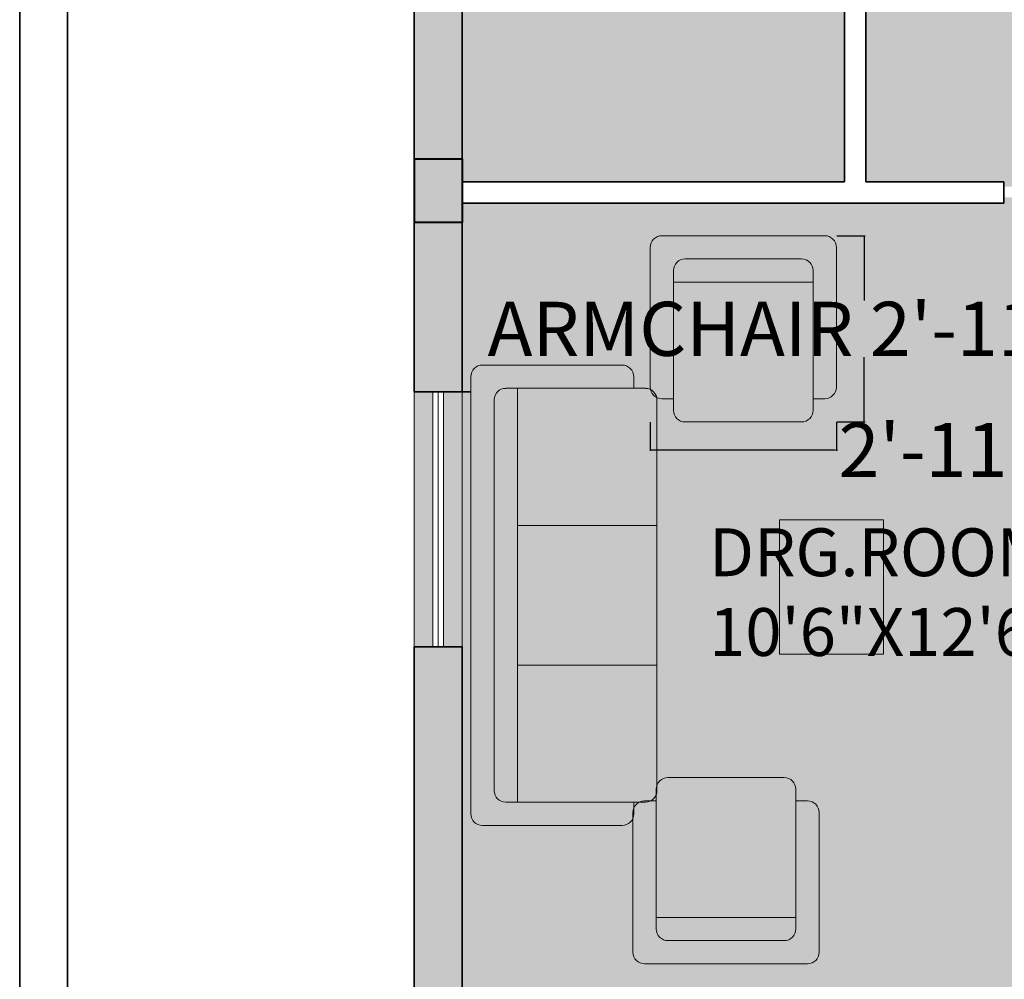
# Model space of a CAD drawing. Units: inches. Extents: x 1077 to 2505, y 1892 to 2728.
# Tile 3 of 26: x 1104 to 1290, y 2157 to 2338. Entities that reach past the tile are written whole.
import ezdxf

# ---------------------------------------------------------------- set-up
doc = ezdxf.new("R2010")
doc.units = ezdxf.units.IN
doc.linetypes.add('ACAD_ISO02W100', pattern=[15, 12, -3])
doc.layers.get('Defpoints').update_dxf_attribs({"color": 220, "linetype": 'ACAD_ISO02W100'})
for name, color, linetype, lineweight in [('00 FURNITURE', 15, 'Continuous', 15), ('A-ANNO-DIMS', 2, 'Continuous', 18), ('A-ANNO-TTLB', 7, 'Continuous', 35), ('A-AREA-IDEN', 7, 'Continuous', 18), ('A-COLS', 7, 'Continuous', 40), ('A-WALL-PATT', 7, 'Continuous', 9), ('WALL', 7, 'Continuous', 35), ('WINDOW', 160, 'Continuous', 13)]:
    doc.layers.add(name, color=color, linetype=linetype, lineweight=lineweight)
doc.layers.add('A-FLOR-PATT', color=254, linetype='Continuous', lineweight=9, true_color=0xd7ebd2)
doc.styles.get("Standard").update_dxf_attribs({"font": 'arial.ttf'})
doc.dimstyles.get("Standard").update_dxf_attribs({"dimtxt": 10.18, "dimasz": 0.18, "dimexe": 0.18, "dimexo": 0.0625, "dimgap": 0.09, "dimtad": 0, "dimtih": 1, "dimtoh": 1, "dimdec": 0, "dimzin": 0, "dimdsep": 46, "dimlunit": 3, "dimtxsty": 'Standard', "dimcen": 0.09, "dimadec": 0, "dimazin": 0, "dimtfac": 1, "dimtdec": 0, "dimtofl": 0, "dimtmove": 0, "dimatfit": 3, "dimfxl": 1, "dimtolj": 1, "dimtzin": 0, "dimarcsym": 0})

# ---------------------------------------------------------------- blocks, each defined once
blk = doc.blocks.new('sofa 6')
for p, q in [((-1044.4, 890), (1044.4, 890)), ((-1100, 166.9), (-1100, 834.3)), ((1100, 834.3), (1100, 166.9)), ((-933.1, 778.7), (933.1, 778.7)), ((-988.8, 55.6), (-988.8, 723.1)), ((988.8, 723.1), (988.8, 55.6)), ((-988.8, 667.5), (988.8, 667.5)), ((-333.8, 667.5), (-333.8, 0)), ((333.7, 667.5), (333.7, 0)), ((-988.8, 111.2), (-1044.4, 111.2)), ((1044.4, 111.2), (988.8, 111.2)), ((933.1, 0), (-933.1, 0))]:
    blk.add_line(p, q)
for centre, start, end in [((-1044.4, 834.3), 90, 180), ((1044.4, 834.3), 0, 90), ((-933.1, 723.1), 90, 180), ((933.1, 723.1), 0, 90), ((-1044.4, 166.9), 180, 270), ((1044.4, 166.9), 270, 0), ((-933.1, 55.6), 180, 270), ((933.1, 55.6), 270, 0)]:
    blk.add_arc(centre, 55.6, start, end)
blk = doc.blocks.new('C1')
h = blk.add_hatch(color=256)
h.dxf.hatch_style = 1
h.paths.add_polyline_path([(1668.56, 2445.41), (1677.56, 2445.41), (1677.56, 2457.41), (1668.56, 2457.41)])
for p, q in [((1668.56, 2457.41), (1677.56, 2457.41)), ((1668.56, 2445.41), (1668.56, 2457.41)), ((1677.56, 2457.41), (1677.56, 2445.41)), ((1677.56, 2445.41), (1668.56, 2445.41))]:
    blk.add_line(p, q)
blk = doc.blocks.new('LOUNGE-ARMCHAIR')
for p, q in [((2.19, 35.04), (32.85, 35.04)), ((0, 6.57), (0, 32.85)), ((35.04, 32.85), (35.04, 6.57)), ((6.57, 30.66), (28.47, 30.66)), ((4.38, 2.19), (4.38, 28.47)), ((30.66, 28.47), (30.66, 2.19)), ((4.38, 26.28), (30.66, 26.28)), ((4.38, 4.38), (2.19, 4.38)), ((32.85, 4.38), (30.66, 4.38)), ((28.47, 0), (6.57, 0))]:
    blk.add_line(p, q)
for centre, start, end in [((2.19, 32.85), 90, 180), ((32.85, 32.85), 0, 90), ((6.57, 28.47), 90, 180), ((28.47, 28.47), 0, 90), ((2.19, 6.57), 180, 270), ((32.85, 6.57), 270, 0), ((6.57, 2.19), 180, 270), ((28.47, 2.19), 270, 0)]:
    blk.add_arc(centre, 2.19, start, end)
blk = doc.blocks.new('WINDOW-48-EXT')
for p, q in [((0, 48), (0, 0)), ((3.5, 48), (3.5, 0)), ((4.5, 48), (4.5, 0)), ((5.5, 48), (5.5, 0)), ((9, 0), (9, 48))]:
    blk.add_line(p, q)
blk = doc.blocks.new('SHEET-FRAME-RESIDENTIAL')
for points in [[(0, 830.04), (543.52, 830.04), (543.52, 0), (0, 0)], [(9, 821.04), (534.52, 821.04), (534.52, 9), (9, 9)]]:
    blk.add_lwpolyline(points, close=True)
blk = doc.blocks.new('*D38')
at = {"layer": 'A-ANNO-DIMS', "color": 0, "lineweight": -2, "transparency": 16777216}
for p, q in [((1258.04, 2297.01), (1263.41, 2297.01)), ((1263.23, 2296.83), (1263.23, 2284.84)), ((1263.23, 2262.15), (1263.23, 2274.13)), ((1258.04, 2261.97), (1263.41, 2261.97))]:
    blk.add_line(p, q, dxfattribs=at)
at = {"layer": 'A-ANNO-DIMS', "color": 0, "transparency": 16777216}
for points in [[(1263.2, 2296.83), (1263.26, 2296.83), (1263.23, 2297.01)], [(1263.2, 2262.15), (1263.26, 2262.15), (1263.23, 2261.97)]]:
    blk.add_solid(points, dxfattribs=at)
at = {"layer": 'Defpoints', "color": 0, "transparency": 16777216}
for p in [(1257.98, 2297.01), (1263.23, 2297.01), (1257.98, 2261.97)]:
    blk.add_point(p, dxfattribs=at)
at = {"layer": 'A-ANNO-DIMS', "color": 0, "transparency": 16777216, "insert": (1263.23, 2279.49), "char_height": 10.18, "attachment_point": 5}
blk.add_mtext('\\A1;ARMCHAIR 2\'-11" TYP.', dxfattribs=at)
blk = doc.blocks.new('*D39')
at = {"layer": 'A-ANNO-DIMS', "color": 0, "lineweight": -2, "transparency": 16777216}
for p, q in [((1222.94, 2261.91), (1222.94, 2256.53)), ((1257.98, 2261.91), (1257.98, 2256.53)), ((1223.12, 2256.71), (1257.8, 2256.71)), ((1257.98, 2256.71), (1258.16, 2256.71))]:
    blk.add_line(p, q, dxfattribs=at)
at = {"layer": 'A-ANNO-DIMS', "color": 0, "transparency": 16777216}
for points in [[(1223.12, 2256.74), (1223.12, 2256.68), (1222.94, 2256.71)], [(1257.8, 2256.74), (1257.8, 2256.68), (1257.98, 2256.71)]]:
    blk.add_solid(points, dxfattribs=at)
at = {"layer": 'Defpoints', "color": 0, "transparency": 16777216}
for p in [(1222.94, 2261.97), (1257.98, 2261.97), (1257.98, 2256.71)]:
    blk.add_point(p, dxfattribs=at)
at = {"layer": 'A-ANNO-DIMS', "color": 0, "transparency": 16777216, "insert": (1293.31, 2256.71), "char_height": 10.18, "attachment_point": 5}
blk.add_mtext('\\A1;2\'-11" TYP.', dxfattribs=at)

msp = doc.modelspace()

# ---------------------------------------------------------------- hatches: boundary and pattern name
at = {"layer": 'A-FLOR-PATT', "transparency": 33554559}
h = msp.add_hatch(color=256, dxfattribs=at)
h.dxf.hatch_style = 1
h.paths.add_polyline_path([(1395.53, 2577.16), (1374.83, 2577.16), (1350.83, 2577.19), (1350.83, 2577.16), (1329.53, 2577.16), (1329.53, 2480.16), (1329.53, 2469.16), (1325.53, 2469.16), (1325.53, 2515.13), (1307.53, 2515.13), (1307.53, 2577.16), (1269.31, 2577.16), (1221.31, 2577.15), (1221.31, 2577.16), (1187.53, 2577.16), (1187.53, 2433.16), (1289.53, 2433.16), (1289.53, 2429.16), (1263.53, 2429.16), (1187.53, 2429.16), (1187.53, 2395.02), (1187.53, 2395.02), (1187.53, 2371.02), (1187.53, 2371.02), (1187.53, 2307.16), (1259.53, 2307.16), (1259.53, 2399.16), (1263.53, 2399.16), (1263.53, 2307.16), (1289.53, 2307.16), (1289.53, 2306.23), (1325.53, 2306.23), (1325.53, 2307.16), (1329.53, 2307.16), (1329.53, 2306.23), (1365.53, 2306.23), (1365.53, 2307.16), (1432.53, 2307.16), (1432.53, 2088.16), (1547.53, 2088.16), (1547.53, 2140.08), (1511.53, 2140.08), (1511.53, 2267.16), (1475.53, 2267.16), (1475.53, 2303.16), (1468.53, 2303.16), (1468.53, 2307.16), (1547.53, 2307.16), (1547.53, 2348.22), (1547.53, 2396.22), (1547.53, 2429.16), (1435.53, 2429.16), (1435.53, 2433.16), (1476.35, 2433.16), (1476.35, 2451.18), (1547.53, 2451.18), (1547.53, 2577.16), (1499.53, 2577.16), (1499.53, 2586.16), (1547.53, 2586.16), (1547.53, 2642.16), (1518.18, 2642.16), (1518.18, 2642.05), (1494.15, 2642.05), (1494.15, 2642.16), (1469.53, 2642.16), (1469.53, 2577.16), (1399.53, 2577.16), (1399.53, 2429.16), (1325.53, 2429.16), (1325.53, 2433.16), (1329.53, 2433.16), (1395.53, 2433.16), (1395.53, 2480.16), (1359.53, 2480.16), (1359.53, 2484.16), (1395.53, 2484.16)])
h.paths.add_polyline_path([(1357.65, 2482.07), (1355.65, 2482.07), (1355.65, 2481.07, 0.414214), (1356.65, 2480.07), (1344.65, 2480.07), (1344.65, 2477.06), (1343.27, 2477.06), (1343.27, 2480.07), (1330.65, 2480.07, -0.414214), (1329.65, 2481.07), (1329.65, 2484.07), (1331.65, 2484.07), (1331.65, 2510.07, -0.446908)], flags=16)
h.paths.add_polyline_path([(1305.09, 2559.18), (1288.89, 2559.18), (1288.89, 2575.38), (1305.09, 2575.38)], flags=16)
h.paths.add_polyline_path([(1304.19, 2560.08), (1289.79, 2560.08), (1289.79, 2574.48), (1304.19, 2574.48)], flags=0)
h.paths.add_polyline_path([(1287.99, 2500.68, -0.414214), (1287.09, 2499.78), (1265.14, 2499.78), (1224.09, 2499.78, -0.414214), (1223.19, 2500.68), (1223.19, 2557.16), (1223.19, 2571.74), (1223.19, 2575.38), (1287.99, 2575.38), (1287.99, 2571.74), (1287.09, 2571.74, -0.414214), (1287.99, 2570.84)], flags=16)
h.paths.add_polyline_path([(1292.98, 2569.05, -1), (1300.92, 2569.05, -1)], flags=0)
h.paths.add_polyline_path([(1293.32, 2569.05, -1), (1300.58, 2569.05, -1)], flags=0)
h.paths.add_polyline_path([(1322.8, 2462.21), (1322.8, 2431.71), (1323.05, 2430.71), (1323.05, 2431.71), (1321.8, 2431.71), (1321.8, 2462.19, 0.404641), (1292.3, 2431.71), (1292.05, 2430.71, -0.414214), (1291.55, 2430.21), (1291.05, 2430.21), (1291.05, 2429.71, -0.414214), (1290.55, 2429.21), (1289.55, 2429.21), (1289.55, 2434.21), (1290.55, 2434.21, -0.414214), (1291.05, 2433.71), (1291.05, 2433.21), (1291.55, 2433.21, -0.414214), (1292.05, 2432.71), (1292.3, 2431.71, -0.414214)], flags=16)
h.paths.add_polyline_path([(1287.82, 2548.28, 0.292232), (1279.17, 2536.8, 0.052719), (1223.93, 2548.28), (1223.28, 2548.28), (1223.28, 2557.16), (1223.93, 2557.16), (1245.42, 2557.16, -0.117785), (1245.77, 2557.93, -0.059418), (1254.87, 2567.02, -0.379859), (1257.28, 2566.88, -0.02509), (1261.41, 2563.32, -0.025935), (1265.65, 2567.02, -0.379859), (1268.06, 2566.88, -0.061767), (1277.52, 2557.43, -0.069393), (1277.82, 2557.16), (1287.82, 2557.16)], flags=0)
h.paths.add_polyline_path([(1263.47, 2548.28), (1260.56, 2548.28, -0.015371), (1258.01, 2546.13, -0.429576), (1255.37, 2546.06, -0.016036), (1252.69, 2548.28), (1223.28, 2548.28), (1223.28, 2554.42), (1246.78, 2554.42, 0.055344), (1255.37, 2546.06, 0.331768), (1257.52, 2545.74, 0.027343), (1262, 2549.64, 0.00919)], flags=0)
h.paths.add_polyline_path([(1295.56, 2568.34), (1296.87, 2569.09), (1296.87, 2570.6, 0.399698), (1295.39, 2569.05, 0.119004)], flags=0)
h.paths.add_polyline_path([(1295.21, 2569.05, -1), (1298.68, 2569.05, -1)], flags=0)
h.paths.add_polyline_path([(1296.95, 2568.96), (1297.03, 2569), (1297.03, 2569.09), (1296.99, 2569.11), (1296.91, 2568.98)], flags=0)
h.paths.add_polyline_path([(1402.28, 2462.19, -0.414214), (1432.78, 2431.69), (1433.03, 2432.69), (1432.78, 2431.69, 0.404641), (1403.28, 2462.17), (1403.28, 2431.69), (1402.03, 2431.69), (1402.03, 2430.69, -0.414214), (1401.53, 2430.19), (1401.03, 2430.19), (1401.03, 2429.69, -0.414214), (1400.53, 2429.19), (1399.53, 2429.19), (1399.53, 2434.19), (1400.53, 2434.19, -0.414214), (1401.03, 2433.69), (1401.03, 2433.19), (1401.53, 2433.19, -0.414214), (1402.03, 2432.69)], flags=16)
h.paths.add_polyline_path([(1470.16, 2535.21, -0.414214), (1471.06, 2536.11), (1527.54, 2536.11), (1542.12, 2536.11), (1545.76, 2536.11), (1545.76, 2471.31), (1542.12, 2471.31), (1542.12, 2472.21, -0.414214), (1541.22, 2471.31), (1471.06, 2471.31, -0.414214), (1470.16, 2472.21), (1470.16, 2494.16)], flags=16)
h.paths.add_polyline_path([(1483.07, 2536.11, 0.253465), (1480.11, 2526.15, 0.2538), (1470.15, 2523.19)], flags=16)
h.paths.add_polyline_path([(1223.19, 2512.69, 0.253465), (1233.14, 2509.74, 0.2538), (1236.1, 2499.77)], flags=16)
h.paths.add_polyline_path([(1469.77, 2578.72), (1469.77, 2581.72), (1471.77, 2581.72), (1471.77, 2607.72, -0.01951), (1473.77, 2607.68), (1473.77, 2579.72), (1473.77, 2578.72, -0.414214), (1472.77, 2577.72), (1470.77, 2577.72, -0.414214)], flags=16)
h.paths.add_polyline_path([(1382.46, 2398.13), (1395.04, 2398.13), (1395.04, 2399.74), (1382.46, 2399.74)], flags=16)
h.paths.add_polyline_path([(1379.94, 2397.18), (1379.94, 2389.82), (1380.5, 2389.82), (1380.5, 2396.05, -0.41429), (1381.06, 2396.61), (1396.47, 2396.61, -0.414213), (1397.03, 2396.05), (1397.03, 2389.82), (1397.59, 2389.82), (1397.59, 2397.18)], flags=16)
h.paths.add_polyline_path([(1263.37, 2428.14), (1263.37, 2426.14, -0.414214), (1262.37, 2425.14), (1261.37, 2425.14), (1233.41, 2425.14, 0.400854), (1259.37, 2401.04), (1259.37, 2401.14), (1261.37, 2401.14, -0.446908), (1233.37, 2427.14), (1259.37, 2427.14), (1259.37, 2429.14), (1262.37, 2429.14, -0.414214)], flags=16)
h.paths.add_polyline_path([(1404.79, 2398.13), (1417.37, 2398.13), (1417.37, 2399.74), (1404.79, 2399.74)], flags=16)
h.paths.add_polyline_path([(1402.27, 2397.18), (1404.79, 2398.13), (1417.37, 2398.13), (1419.92, 2397.18)], flags=16)
h.paths.add_polyline_path([(1432.26, 2383.16), (1432.26, 2370.59), (1433.87, 2370.59), (1433.87, 2383.16)], flags=16)
h.paths.add_polyline_path([(1431.3, 2385.69), (1423.84, 2385.69), (1423.84, 2385.13), (1430.18, 2385.13, -0.41429), (1430.74, 2384.57), (1430.74, 2369.16, -0.414237), (1430.18, 2368.6), (1423.84, 2368.6), (1423.84, 2368.03), (1431.3, 2368.03)], flags=16)
h.paths.add_polyline_path([(1417.37, 2351.16), (1417.37, 2349.54), (1418.9, 2349.54, 0.414236), (1419.92, 2350.56), (1419.92, 2352.11)], flags=16)
h.paths.add_polyline_path([(1395.04, 2351.16), (1395.04, 2349.54), (1396.58, 2349.54, 0.414235), (1397.59, 2350.56), (1397.59, 2352.11)], flags=16)
h.paths.add_polyline_path([(1366.7, 2370.05), (1365.09, 2370.05), (1365.09, 2368.52, 0.414235), (1366.11, 2367.5), (1367.66, 2367.5)], flags=16)
h.paths.add_polyline_path([(1419.36, 2359.47), (1419.36, 2353.24, -0.41419), (1418.8, 2352.68), (1403.39, 2352.68, -0.414137), (1402.83, 2353.24), (1402.83, 2359.47), (1397.03, 2359.47), (1397.03, 2353.24, -0.414189), (1396.47, 2352.68), (1381.06, 2352.68, -0.414137), (1380.5, 2353.24), (1380.5, 2359.47)], flags=16)
h.paths.add_polyline_path([(1222.29, 2559.18), (1206.09, 2559.18), (1206.09, 2575.38), (1222.29, 2575.38)], flags=16)
h.paths.add_polyline_path([(1221.39, 2560.08), (1206.99, 2560.08), (1206.99, 2574.48), (1221.39, 2574.48)], flags=0)
h.paths.add_polyline_path([(1482, 2577.72), (1482, 2580.73), (1483.38, 2580.73), (1483.38, 2577.72), (1484.77, 2577.72), (1484.77, 2574.72), (1483.38, 2574.72), (1483.38, 2577.72)], flags=16)
h.paths.add_polyline_path([(1266.37, 2415.53), (1266.37, 2414.14), (1263.37, 2414.14), (1263.37, 2415.53), (1260.36, 2415.53), (1260.36, 2416.91), (1263.37, 2416.91), (1263.37, 2415.53)], flags=16)
h.paths.add_polyline_path([(1210.26, 2569.05, -1), (1218.19, 2569.05, -1)], flags=0)
h.paths.add_polyline_path([(1210.6, 2569.05, -1), (1217.85, 2569.05, -1)], flags=0)
h.paths.add_polyline_path([(1212.84, 2568.34), (1214.15, 2569.09), (1214.15, 2570.6, 0.399698), (1212.67, 2569.05, 0.119004)], flags=0)
h.paths.add_polyline_path([(1212.49, 2569.05, -1), (1215.96, 2569.05, -1)], flags=0)
h.paths.add_polyline_path([(1214.23, 2568.96), (1214.3, 2568.91), (1214.3, 2569)], flags=0)
h.paths.add_polyline_path([(1507.18, 2480.12, 0.052719), (1518.66, 2535.36), (1518.66, 2536.01), (1527.54, 2536.01), (1527.54, 2535.36), (1527.54, 2513.88, -0.117785), (1528.31, 2513.53, -0.059418), (1537.4, 2504.43, -0.379859), (1537.26, 2502.01, -0.02509), (1533.7, 2497.89, -0.025935), (1537.4, 2493.64, -0.379859), (1537.26, 2491.23, -0.061767), (1527.8, 2481.77, -0.069393), (1527.54, 2481.47), (1527.54, 2471.47), (1518.66, 2471.47, 0.292232)], flags=0)
h.paths.add_polyline_path([(1516.43, 2503.92, -0.016036), (1518.66, 2506.6), (1518.66, 2536.01), (1524.8, 2536.01), (1524.8, 2512.51, 0.055344), (1516.43, 2503.92, 0.331768), (1516.12, 2501.77, 0.027343), (1520.01, 2497.29, 0.00919), (1518.66, 2495.82), (1518.66, 2498.73, -0.015371), (1516.5, 2501.28, -0.429576)], flags=0)
h.paths.add_polyline_path([(1499.63, 2625.5, -0.171636), (1502.82, 2631.01), (1502.82, 2633.37), (1498.68, 2633.37, -0.414214), (1497.7, 2634.36), (1497.7, 2640.66, -0.414214), (1498.68, 2641.64), (1514.82, 2641.64, -0.414214), (1515.81, 2640.66), (1515.81, 2634.36, -0.414214), (1514.82, 2633.37), (1510.69, 2633.37), (1510.69, 2631.01, -0.171636), (1513.88, 2625.5, -0.258205), (1509.31, 2614.47), (1504.19, 2614.47, -0.258205)], flags=16)
h.paths.add_polyline_path([(1501.2, 2625.5, -0.171636), (1504.39, 2631.01), (1509.12, 2631.01, -0.171636), (1512.3, 2625.5, -0.210384), (1509.35, 2616.02), (1504.16, 2616.02, -0.210384)], flags=0)
h.paths.add_polyline_path([(1529.56, 2537.01), (1529.56, 2553.21), (1545.76, 2553.21), (1545.76, 2537.01)], flags=16)
h.paths.add_polyline_path([(1530.46, 2537.91), (1530.46, 2552.31), (1544.86, 2552.31), (1544.86, 2537.91)], flags=0)
h.paths.add_polyline_path([(1535.45, 2545.07, -1), (1543.39, 2545.07, -1)], flags=0)
h.paths.add_polyline_path([(1535.8, 2545.07, -1), (1543.05, 2545.07, -1)], flags=0)
h.paths.add_polyline_path([(1529.56, 2470.41), (1545.76, 2470.41), (1545.76, 2454.21), (1529.56, 2454.21)], flags=16)
h.paths.add_polyline_path([(1541.16, 2544.99), (1540.98, 2544.99, -0.544606), (1538.71, 2543.68), (1538.62, 2543.53, 0.547962)], flags=0)
h.paths.add_polyline_path([(1530.46, 2469.51), (1544.86, 2469.51), (1544.86, 2455.11), (1530.46, 2455.11)], flags=0)
h.paths.add_polyline_path([(1539.47, 2545.14), (1539.42, 2545.22), (1539.38, 2545.14)], flags=0)
h.paths.add_polyline_path([(1543.39, 2462.34, -1), (1535.45, 2462.34, -1)], flags=0)
h.paths.add_polyline_path([(1543.05, 2462.34, -1), (1535.8, 2462.34, -1)], flags=0)
h.paths.add_polyline_path([(1541.16, 2462.27), (1540.98, 2462.27, -0.544606), (1538.71, 2460.96), (1538.62, 2460.8, 0.547962)], flags=0)
h.paths.add_polyline_path([(1539.47, 2462.42), (1539.42, 2462.5), (1539.38, 2462.42)], flags=0)
h.paths.add_polyline_path([(1435.32, 2335.25, -0.414214), (1465.82, 2304.75), (1466.07, 2305.75), (1465.82, 2304.75, 0.404641), (1436.32, 2335.23), (1436.32, 2304.75), (1435.07, 2304.75), (1435.07, 2303.75, -0.414214), (1434.57, 2303.25), (1434.07, 2303.25), (1434.07, 2302.75, -0.414214), (1433.57, 2302.25), (1432.57, 2302.25), (1432.57, 2307.25), (1433.57, 2307.25, -0.414214), (1434.07, 2306.75), (1434.07, 2306.25), (1434.57, 2306.25, -0.414214), (1435.07, 2305.75)], flags=16)
h.paths.add_polyline_path([(1532.13, 2635.71), (1535.43, 2635.71), (1535.43, 2635.89), (1532.13, 2635.89)], flags=16)
edge = h.paths.add_edge_path(flags=16)
edge.add_arc((1535.98, 2632.67), 0.183, 270, 360)
edge.add_line((1536.17, 2632.67), (1536.17, 2639.82))
edge.add_line((1536.17, 2639.82), (1538.29, 2639.82))
edge.add_line((1538.29, 2639.82), (1538.29, 2641.82))
edge.add_line((1538.29, 2641.82), (1533.25, 2641.82))
edge.add_line((1533.25, 2641.82), (1533.25, 2639.82))
edge.add_line((1533.25, 2639.82), (1534.87, 2639.82))
edge.add_line((1534.87, 2639.82), (1534.87, 2639))
edge.add_line((1534.87, 2639), (1533.7, 2639))
edge.add_line((1533.7, 2639), (1533.7, 2639.82))
edge.add_line((1533.7, 2639.82), (1533.25, 2639.82))
edge.add_line((1533.25, 2639.82), (1533.25, 2641.82))
edge.add_line((1533.25, 2641.82), (1538.29, 2641.82))
edge.add_line((1538.29, 2641.82), (1538.29, 2641.34))
edge.add_line((1538.29, 2641.34), (1540.64, 2641.58))
edge.add_line((1540.64, 2641.58), (1540.64, 2641.82))
edge.add_line((1540.64, 2641.82), (1541.5, 2641.82))
edge.add_line((1541.5, 2641.82), (1541.5, 2641.25))
edge.add_line((1541.5, 2641.25), (1541.31, 2639.79))
edge.add_ellipse((1541.09, 2638.95), major_axis=(-1.08, 0), ratio=0.790849, start_angle=180, end_angle=255.2976, ccw=False)
edge.add_line((1542.17, 2638.95), (1542.17, 2638.38))
edge.add_ellipse((1541.09, 2638.38), major_axis=(-1.08, 0), ratio=0.790849, start_angle=0, end_angle=180, ccw=False)
edge.add_line((1540, 2638.38), (1540.01, 2638.87))
edge.add_ellipse((1541.09, 2638.95), major_axis=(-1.08, 0), ratio=0.790849, start_angle=284.7024, end_angle=364.0401, ccw=False)
edge.add_line((1540.78, 2639.75), (1540.78, 2641.25))
edge.add_line((1540.78, 2641.25), (1540.64, 2641.25))
edge.add_line((1540.64, 2641.25), (1538.29, 2641.01))
edge.add_line((1538.29, 2641.01), (1538.29, 2639.82))
edge.add_line((1538.29, 2639.82), (1536.17, 2639.82))
edge.add_line((1536.17, 2639.82), (1536.17, 2632.48))
edge.add_line((1536.17, 2632.48), (1535.98, 2632.48))
h.paths.add_polyline_path([(1496.32, 2250.34, -0.292371), (1498.9, 2247.83, -0.085148), (1501.21, 2208.85, -0.01331), (1500.27, 2098.5, -0.379287), (1497.22, 2095.28, -0.0502), (1441.54, 2095.28, -0.379287), (1438.5, 2098.5, -0.01331), (1437.56, 2208.85, -0.086132), (1439.96, 2248.26, -0.295116), (1442.59, 2250.78, -0.114238)], flags=16)
h.paths.add_polyline_path([(1495.16, 2205.84, -0.355389), (1496.7, 2202.1), (1492.94, 2189.65, -0.398275), (1489.12, 2187.47, 0.113332), (1449.64, 2187.47, -0.398275), (1445.82, 2189.65), (1442.06, 2202.1, -0.355394), (1443.6, 2205.84, -0.265725)], flags=0)
h.paths.add_polyline_path([(1440.37, 2195.72), (1445.94, 2181.67), (1445.94, 2160.63), (1440.84, 2157.26)], flags=0)
h.paths.add_polyline_path([(1498.46, 2195.72), (1497.99, 2157.26), (1492.88, 2160.63), (1492.88, 2181.67)], flags=0)
h.paths.add_polyline_path([(1445.94, 2158.37), (1445.94, 2137.12), (1441.12, 2122.56), (1440.87, 2155.03)], flags=0)
h.paths.add_polyline_path([(1492.88, 2158.37), (1497.96, 2155.03), (1497.71, 2122.56), (1492.88, 2137.12)], flags=0)
h.paths.add_polyline_path([(1489.88, 2130.4), (1494.39, 2107.67, -0.090102), (1444.44, 2107.65), (1448.95, 2130.39, 0.036636)], flags=0)
h.paths.add_polyline_path([(1447.54, 2159.34), (1497.44, 2159.34), (1497.44, 2177.89), (1447.54, 2177.89)], flags=8)
h.paths.add_polyline_path([(1196.44, 2354.84), (1246.65, 2354.84), (1246.65, 2388.43), (1196.44, 2388.43)], flags=24)
h.paths.add_polyline_path([(1296.09, 2360.25), (1353.81, 2360.25), (1353.81, 2393.84), (1296.09, 2393.84)], flags=24)
h.paths.add_polyline_path([(1400.72, 2471.85), (1470.63, 2471.85), (1470.63, 2505.44), (1400.72, 2505.44)], flags=24)
h.paths.add_polyline_path([(1324.78, 2448.48), (1394.95, 2448.48), (1394.95, 2467.02), (1324.78, 2467.02)], flags=24)
h.paths.add_polyline_path([(1335.08, 2531.43), (1389.67, 2531.43), (1389.67, 2565.02), (1335.08, 2565.02)], flags=24)
h.paths.add_polyline_path([(1225.76, 2460), (1295.67, 2460), (1295.67, 2493.58), (1225.76, 2493.58)], flags=24)
h = msp.add_hatch(color=256, dxfattribs=at)
h.dxf.hatch_style = 1
h.paths.add_polyline_path([(1547.53, 2348.22), (1547.53, 2396.22), (1547.53, 2425.11), (1547.53, 2425.11), (1547.53, 2429.16), (1435.53, 2429.16), (1434.03, 2429.21), (1434.03, 2430.19), (1433.03, 2430.19), (1432.78, 2431.69, 0.404641), (1403.28, 2462.17), (1403.28, 2431.69), (1402.03, 2431.69), (1402.03, 2430.19), (1401.03, 2430.19), (1401.03, 2429.19), (1399.53, 2429.19), (1399.53, 2429.19), (1399.53, 2429.16), (1334.67, 2429.16), (1334.67, 2423.95), (1325.67, 2423.95), (1325.67, 2429.16), (1325.53, 2429.16), (1324.05, 2429.24), (1324.05, 2430.21), (1323.05, 2430.21), (1323.05, 2431.71), (1321.8, 2431.71), (1321.8, 2462.19, 0.416544), (1292.05, 2430.73, -0.423614), (1291.55, 2430.21), (1291.05, 2430.21), (1291.05, 2429.21), (1289.55, 2429.21), (1289.53, 2429.21), (1289.53, 2429.16), (1263.37, 2429.16), (1263.37, 2415.53), (1266.37, 2415.53), (1266.37, 2414.14), (1263.37, 2414.14), (1263.37, 2399.16), (1263.53, 2399.16), (1263.53, 2307.16), (1289.53, 2307.16), (1289.53, 2306.23), (1323.26, 2306.23), (1323.26, 2307.21), (1332.26, 2307.21), (1365.53, 2306.23), (1365.53, 2307.16), (1432.53, 2307.16), (1432.57, 2307.16), (1432.57, 2307.25), (1434.07, 2307.25), (1434.07, 2306.25), (1435.32, 2306.25), (1435.32, 2335.25, -0.407346), (1466.07, 2305.73, -0.423614), (1466.57, 2306.25), (1467.07, 2306.25), (1467.07, 2307.25), (1468.57, 2307.25), (1547.53, 2307.16), (1547.53, 2307.2)])
h.paths.add_polyline_path([(1430.74, 2369.16), (1430.74, 2384.57, 0.41429), (1430.18, 2385.13), (1423.84, 2385.13), (1423.84, 2368.6), (1430.18, 2368.6, 0.414237)], flags=16)
h.paths.add_polyline_path([(1432.26, 2383.16), (1432.26, 2370.59), (1433.87, 2370.59), (1433.87, 2383.16)], flags=16)
h.paths.add_polyline_path([(1431.3, 2368.03), (1431.3, 2385.69), (1432.26, 2383.16), (1432.26, 2370.59)], flags=16)
h.paths.add_polyline_path([(1417.37, 2351.16), (1417.37, 2349.54), (1418.9, 2349.54, 0.414236), (1419.92, 2350.56), (1419.92, 2352.11)], flags=16)
h.paths.add_polyline_path([(1403.39, 2352.68), (1418.78, 2352.68, 0.42427), (1419.36, 2353.24), (1419.36, 2359.47), (1402.83, 2359.47), (1402.83, 2353.24, 0.414137)], flags=16)
h.paths.add_polyline_path([(1366.7, 2370.05), (1365.09, 2370.05), (1365.09, 2368.52, 0.414235), (1366.11, 2367.5), (1367.66, 2367.5)], flags=16)
h.paths.add_polyline_path([(1382.46, 2398.13), (1395.04, 2398.13), (1395.04, 2399.74), (1382.46, 2399.74)], flags=16)
h.paths.add_polyline_path([(1396.47, 2396.61), (1381.06, 2396.61, 0.41429), (1380.5, 2396.05), (1380.5, 2389.82), (1397.03, 2389.82), (1397.03, 2396.05, 0.414213)], flags=16)
h.paths.add_polyline_path([(1402.27, 2397.18), (1402.83, 2396.05, -0.414213), (1403.39, 2396.61)], flags=16)
h.paths.add_polyline_path([(1418.8, 2396.61), (1419.36, 2396.61), (1419.36, 2396.05, 0.414237)], flags=16)
h.paths.add_polyline_path([(1404.79, 2398.13), (1417.37, 2398.13), (1417.37, 2399.74), (1404.79, 2399.74)], flags=16)
h.paths.add_polyline_path([(1381.06, 2352.68, -0.414213), (1380.5, 2353.24), (1380.27, 2352.11)], flags=16)
h.paths.add_polyline_path([(1396.58, 2349.54), (1396.58, 2349.54), (1395.04, 2349.54), (1395.04, 2349.54), (1382.46, 2349.54), (1382.46, 2351.16), (1395.04, 2351.16), (1397.59, 2352.11), (1397.59, 2350.56, -0.414235)], flags=16)
h.paths.add_polyline_path([(1379.94, 2397.18), (1382.46, 2398.13), (1395.04, 2398.13), (1397.59, 2397.18)], flags=16)
h.paths.add_polyline_path([(1368.78, 2384.59, 0.414213), (1368.22, 2384.03), (1367.66, 2367.5), (1367.66, 2385.15)], flags=16)
h.paths.add_polyline_path([(1547.53, 2574.38), (1547.51, 2574.38), (1547.51, 2577.16), (1499.53, 2577.16), (1484.77, 2577.44), (1484.77, 2574.72), (1483.38, 2574.72), (1483.38, 2577.72), (1482, 2577.72), (1469.53, 2577.72), (1469.53, 2577.16), (1401.95, 2577.16), (1401.95, 2574.12), (1399.53, 2574.12), (1399.53, 2434.19), (1401.03, 2434.19), (1401.03, 2433.19), (1402.28, 2433.19), (1402.28, 2462.19, -0.407346), (1433.03, 2432.67, -0.423614), (1433.53, 2433.19), (1434.03, 2433.19), (1434.03, 2434.19), (1435.53, 2434.19), (1476.35, 2433.81), (1476.35, 2451.18), (1547.53, 2451.18)])
h.paths.add_polyline_path([(1470.16, 2535.21, -0.414214), (1471.06, 2536.11), (1527.54, 2536.11), (1542.12, 2536.11), (1545.76, 2536.11), (1545.76, 2471.31), (1542.12, 2471.31), (1542.12, 2472.21, -0.414214), (1541.22, 2471.31), (1471.06, 2471.31, -0.414214), (1470.16, 2472.21), (1470.16, 2494.16)], flags=16)
h.paths.add_polyline_path([(1483.07, 2536.11, 0.253465), (1480.11, 2526.15, 0.2538), (1470.15, 2523.19)], flags=16)
h.paths.add_polyline_path([(1525.55, 2481.52, -0.000893), (1524.8, 2482.24), (1524.8, 2471.47), (1527.54, 2471.47), (1527.54, 2472.12), (1527.54, 2481.47, -0.388819)], flags=0)
h.paths.add_polyline_path([(1518.66, 2536.01), (1527.54, 2536.01), (1527.54, 2535.36), (1527.54, 2513.88, -0.117785), (1528.31, 2513.53, -0.059418), (1537.4, 2504.43, -0.379859), (1537.26, 2502.01, -0.02509), (1533.7, 2497.89, 0.033431), (1528.3, 2502.74, 0.308459), (1526.25, 2502.88, 0.047827), (1518.66, 2495.82), (1518.66, 2498.73, -0.015371), (1516.5, 2501.28, -0.429576), (1516.43, 2503.92, -0.016036), (1518.66, 2506.6)], flags=0)
h.paths.add_polyline_path([(1529.56, 2537.01), (1529.56, 2553.21), (1545.76, 2553.21), (1545.76, 2537.01)], flags=16)
h.paths.add_polyline_path([(1530.46, 2537.91), (1530.46, 2552.31), (1544.86, 2552.31), (1544.86, 2537.91)], flags=0)
h.paths.add_polyline_path([(1535.8, 2545.07, -1), (1543.05, 2545.07, -1)], flags=0)
h.paths.add_polyline_path([(1541.16, 2544.99), (1540.98, 2544.99, -0.544606), (1538.71, 2543.68), (1538.62, 2543.53, 0.547962)], flags=0)
h.paths.add_polyline_path([(1539.47, 2545.14), (1539.42, 2545.22), (1539.38, 2545.14)], flags=0)
h.paths.add_polyline_path([(1529.56, 2470.41), (1545.76, 2470.41), (1545.76, 2454.21), (1529.56, 2454.21)], flags=16)
h.paths.add_polyline_path([(1530.46, 2469.51), (1544.86, 2469.51), (1544.86, 2455.11), (1530.46, 2455.11)], flags=0)
h.paths.add_polyline_path([(1535.8, 2462.34, -1), (1543.05, 2462.34, -1)], flags=0)
h.paths.add_polyline_path([(1541.16, 2462.27), (1540.98, 2462.27, -0.544606), (1538.71, 2460.96), (1538.62, 2460.8, 0.547962)], flags=0)
h.paths.add_polyline_path([(1539.47, 2462.42), (1539.42, 2462.5), (1539.38, 2462.42)], flags=0)
h.paths.add_polyline_path([(1395.53, 2574.12), (1392.95, 2574.12), (1392.95, 2577.16), (1374.83, 2577.16), (1350.83, 2577.19), (1350.83, 2577.16), (1332.07, 2577.16), (1332.07, 2574), (1329.53, 2574), (1329.53, 2484.07), (1331.65, 2484.07), (1331.65, 2510.07, -0.423677), (1357.76, 2484.07), (1359.53, 2484.07), (1359.53, 2484.16), (1395.53, 2484.16)], flags=17)
h.paths.add_polyline_path([(1395.53, 2480.16), (1359.06, 2480.16, 0.437533), (1359.53, 2481.55), (1359.53, 2484.16), (1395.53, 2484.16), (1395.53, 2574.12), (1392.95, 2574.12), (1392.95, 2577.16), (1374.83, 2577.16), (1350.83, 2577.19), (1350.83, 2577.16), (1332.07, 2577.16), (1332.07, 2574), (1329.53, 2574), (1329.53, 2484.07), (1329.65, 2484.07), (1329.65, 2481.07), (1329.53, 2480.16), (1329.53, 2469.16), (1325.53, 2469.16), (1325.53, 2515.13), (1307.53, 2515.13), (1307.53, 2577.16), (1269.31, 2577.16), (1221.31, 2577.15), (1221.31, 2577.16), (1187.61, 2577.16), (1187.61, 2574.03), (1187.53, 2433.16), (1289.55, 2433.16), (1289.55, 2434.21), (1291.05, 2434.21), (1291.05, 2433.21), (1292.05, 2433.21), (1292.3, 2431.71, -0.414214), (1322.8, 2462.21), (1323.05, 2432.71, -0.414214), (1323.55, 2433.21), (1324.05, 2433.21), (1324.05, 2434.21), (1325.67, 2434.21), (1325.67, 2435.95), (1334.67, 2435.95), (1334.67, 2433.16), (1395.53, 2433.16)])
h.paths.add_polyline_path([(1344.65, 2480.07), (1344.65, 2477.06), (1343.27, 2477.06), (1343.27, 2480.07), (1332.65, 2480.07, 0.414214), (1333.65, 2481.07), (1333.65, 2482.07), (1331.65, 2482.07), (1331.65, 2484.07), (1331.65, 2510.07, -0.446908), (1357.65, 2482.07), (1355.65, 2482.07), (1355.65, 2481.07, 0.414214), (1356.65, 2480.07)], flags=16)
h.paths.add_polyline_path([(1287.99, 2500.68, -0.414214), (1287.09, 2499.78), (1265.14, 2499.78), (1224.09, 2499.78, -0.414214), (1223.19, 2500.68), (1223.19, 2557.16), (1223.19, 2571.74), (1223.19, 2575.38), (1287.99, 2575.38), (1287.99, 2571.74), (1287.09, 2571.74, -0.414214), (1287.99, 2570.84)], flags=16)
h.paths.add_polyline_path([(1277.77, 2555.17, -0.000893), (1277.05, 2554.42), (1287.82, 2554.42), (1287.82, 2557.16), (1287.17, 2557.16), (1277.82, 2557.16, -0.388819)], flags=0)
h.paths.add_polyline_path([(1223.28, 2548.28), (1223.28, 2557.16), (1223.93, 2557.16), (1245.42, 2557.16, -0.117785), (1245.77, 2557.93, -0.059418), (1254.87, 2567.02, -0.379859), (1257.28, 2566.88, -0.02509), (1261.41, 2563.32, 0.033431), (1256.55, 2557.93, 0.308459), (1256.41, 2555.88, 0.047827), (1263.47, 2548.28), (1260.56, 2548.28, -0.015371), (1258.01, 2546.13, -0.429576), (1255.37, 2546.06, -0.016036), (1252.69, 2548.28)], flags=0)
h.paths.add_polyline_path([(1305.09, 2559.18), (1288.89, 2559.18), (1288.89, 2575.38), (1305.09, 2575.38)], flags=16)
h.paths.add_polyline_path([(1304.19, 2560.08), (1289.79, 2560.08), (1289.79, 2574.48), (1304.19, 2574.48)], flags=0)
h.paths.add_polyline_path([(1300.58, 2569.05, -1), (1293.32, 2569.05, -1)], flags=0)
h.paths.add_polyline_path([(1223.19, 2512.69, 0.253465), (1233.14, 2509.74, 0.2538), (1236.1, 2499.77)], flags=16)
h.paths.add_polyline_path([(1295.56, 2568.34), (1296.87, 2569.09), (1296.87, 2570.6, 0.399698), (1295.39, 2569.05, 0.119004)], flags=0)
h.paths.add_polyline_path([(1295.21, 2569.05, -1), (1298.68, 2569.05, -1)], flags=0)
h.paths.add_polyline_path([(1296.95, 2568.96), (1297.03, 2569), (1297.03, 2569.09), (1296.99, 2569.11), (1296.91, 2568.98)], flags=0)
h.paths.add_polyline_path([(1222.29, 2559.18), (1206.09, 2559.18), (1206.09, 2575.38), (1222.29, 2575.38)], flags=16)
h.paths.add_polyline_path([(1221.39, 2560.08), (1206.99, 2560.08), (1206.99, 2574.48), (1221.39, 2574.48)], flags=0)
h.paths.add_polyline_path([(1217.85, 2569.05, -1), (1210.6, 2569.05, -1)], flags=0)
h.paths.add_polyline_path([(1212.84, 2568.34), (1214.15, 2569.09), (1214.15, 2570.6, 0.399698), (1212.67, 2569.05, 0.119004)], flags=0)
h.paths.add_polyline_path([(1212.49, 2569.05, -1), (1215.96, 2569.05, -1)], flags=0)
h.paths.add_polyline_path([(1214.23, 2568.96), (1214.3, 2569), (1214.3, 2569.09), (1214.26, 2569.11), (1214.19, 2568.98)], flags=0)
h.paths.add_polyline_path([(1259.53, 2399.14), (1259.37, 2399.14), (1259.37, 2401.04, -0.423677), (1233.37, 2427.14), (1259.37, 2427.14), (1259.37, 2429.16), (1187.53, 2429.16), (1187.53, 2395.02), (1187.53, 2395.02), (1187.53, 2371.02), (1187.53, 2371.02), (1187.53, 2311.49), (1187.55, 2311.49), (1187.55, 2307.16), (1259.53, 2307.16)])
h.paths.add_polyline_path([(1323.26, 2295.21), (1323.26, 2304.23), (1289.53, 2304.23), (1289.53, 2303.16), (1187.55, 2303.16), (1187.55, 2299.49), (1178.53, 2299.49), (1178.53, 2267.66), (1178.53, 2219.66), (1182.03, 2219.66), (1182.03, 2267.67), (1184.03, 2267.67), (1184.03, 2219.66), (1187.53, 2219.66), (1187.53, 2153.16), (1228.13, 2153.16), (1276.13, 2153.16), (1276.13, 2153.16), (1324.54, 2153.16), (1324.54, 2154.67), (1325.54, 2154.67), (1325.54, 2155.92), (1296.54, 2155.92, -0.407346), (1326.06, 2186.67, -0.423614), (1325.54, 2187.17), (1325.54, 2187.67), (1324.54, 2187.67), (1324.54, 2189.17), (1325.43, 2295.21)])
h.paths.add_polyline_path([(1432.53, 2307.16), (1365.53, 2307.16), (1365.53, 2306.23), (1365.53, 2303.16), (1428.53, 2303.16), (1428.53, 2221.2), (1428.57, 2221.2), (1428.57, 2197.2), (1428.53, 2197.16), (1428.53, 2303.01), (1404.46, 2303.01), (1404.46, 2221.2), (1329.53, 2221.2), (1329.53, 2307.16), (1325.53, 2307.16), (1325.53, 2295.21), (1325.43, 2295.21), (1324.54, 2189.17), (1324.54, 2187.67), (1326.04, 2187.67, 1.016365), (1326.06, 2186.67, 0.407348), (1296.54, 2155.92), (1325.54, 2155.92), (1325.54, 2154.67), (1324.54, 2154.67), (1324.54, 2153.16), (1329.53, 2153.16), (1329.53, 2144.16), (1432.53, 2144.16)])
h.paths.add_polyline_path([(1361.95, 2194.26), (1361.95, 2193.16), (1329.53, 2193.16), (1329.53, 2189.16), (1329.54, 2188.17), (1329.54, 2189.16), (1329.53, 2189.16), (1329.53, 2193.16), (1361.95, 2193.16), (1361.95, 2196.26), (1409.95, 2196.26), (1409.95, 2194.26)], flags=16)
h.paths.add_polyline_path([(1377.02, 2200.5), (1345.91, 2200.5), (1345.91, 2218.4), (1347.87, 2218.4), (1347.87, 2219.18), (1374.75, 2219.18), (1374.75, 2218.4), (1377.02, 2218.4)], flags=16)
h.paths.add_polyline_path([(1367.07, 2210.7, -1), (1373.34, 2210.7, -1)], flags=0)
h.paths.add_polyline_path([(1349.92, 2210.7, -1), (1356.98, 2210.7, -1)], flags=0)
h.paths.add_polyline_path([(1405.95, 2256.57), (1405.95, 2277.6), (1427.86, 2277.6), (1427.86, 2256.57)], flags=16)
h.paths.add_polyline_path([(1412.92, 2258.68, -0.414201), (1410.93, 2260.67), (1410.93, 2273.62, -0.414239), (1412.92, 2275.61), (1423.88, 2275.61, -0.414227), (1425.87, 2273.62), (1425.87, 2260.67, -0.414214), (1423.88, 2258.68)], flags=0)
h.paths.add_polyline_path([(1407.61, 2263.66, -1), (1409.18, 2263.66, -1)], flags=0)
h.paths.add_polyline_path([(1407.61, 2267.14, -1), (1409.18, 2267.14, -1)], flags=0)
h.paths.add_polyline_path([(1416.91, 2267.15, -1), (1419.89, 2267.15, -1)], flags=0)
h.paths.add_polyline_path([(1407.61, 2270.63, -1), (1409.18, 2270.63, -1)], flags=0)
h.paths.add_polyline_path([(1475.53, 2303.16), (1468.57, 2303.16), (1468.57, 2302.25), (1467.07, 2302.25), (1467.07, 2303.25), (1466.07, 2303.25), (1465.82, 2304.75, 0.404641), (1436.32, 2335.23), (1436.32, 2304.75), (1435.07, 2304.75), (1435.07, 2303.25), (1434.07, 2303.25), (1434.07, 2302.25), (1432.53, 2302.25), (1432.53, 2144.16), (1432.53, 2088.16), (1547.52, 2088.16), (1547.52, 2100.19), (1547.52, 2140.08), (1511.53, 2140.08), (1511.53, 2267.16), (1475.53, 2267.16)])
h.paths.add_polyline_path([(1438.35, 2102.86, 0.033498), (1438.37, 2102.21, -0.000079)], flags=16)
h.paths.add_polyline_path([(1496.32, 2250.34, -0.292371), (1498.9, 2247.83, -0.085148), (1501.21, 2208.85, -0.012784), (1500.42, 2102.86, -0.033498), (1500.39, 2102.21, 0.012863), (1501.21, 2208.85, 0.077283), (1499.67, 2244.3, 0.265882), (1497.48, 2246.8, 0.14401), (1441.46, 2247.36, 0.270646), (1439.21, 2244.85, -0.007564), (1439.96, 2248.26, -0.295116), (1442.59, 2250.78, -0.114238)], flags=16)
h.paths.add_polyline_path([(1495.16, 2205.84, -0.355389), (1496.7, 2202.1), (1492.94, 2189.65, -0.398275), (1489.12, 2187.47, 0.113332), (1449.64, 2187.47, -0.398275), (1445.82, 2189.65), (1442.06, 2202.1, -0.355394), (1443.6, 2205.84, -0.265725)], flags=16)
h.paths.add_polyline_path([(1440.37, 2195.72), (1445.94, 2181.67), (1445.94, 2160.63), (1440.84, 2157.26)], flags=16)
h.paths.add_polyline_path([(1498.46, 2195.72), (1497.99, 2157.26), (1492.88, 2160.63), (1492.88, 2181.67)], flags=16)
h.paths.add_polyline_path([(1445.94, 2158.37), (1445.94, 2137.12), (1441.12, 2122.56), (1440.87, 2155.03)], flags=16)
h.paths.add_polyline_path([(1492.88, 2158.37), (1497.96, 2155.03), (1497.71, 2122.56), (1492.88, 2137.12)], flags=16)
h.paths.add_polyline_path([(1489.88, 2130.4), (1494.39, 2107.67, -0.090102), (1444.44, 2107.65), (1448.95, 2130.39, 0.036636)], flags=16)
h.paths.add_polyline_path([(1296.09, 2360.25), (1353.81, 2360.25), (1353.81, 2393.84), (1296.09, 2393.84)], flags=24)
h.paths.add_polyline_path([(1400.72, 2471.85), (1470.63, 2471.85), (1470.63, 2505.44), (1400.72, 2505.44)], flags=24)
h.paths.add_polyline_path([(1335.08, 2531.43), (1389.67, 2531.43), (1389.67, 2565.02), (1335.08, 2565.02)], flags=24)
h.paths.add_polyline_path([(1324.78, 2448.48), (1394.95, 2448.48), (1394.95, 2467.02), (1324.78, 2467.02)], flags=24)
h.paths.add_polyline_path([(1225.76, 2460), (1295.67, 2460), (1295.67, 2493.58), (1225.76, 2493.58)], flags=24)
h.paths.add_polyline_path([(1196.44, 2354.84), (1246.65, 2354.84), (1246.65, 2388.43), (1196.44, 2388.43)], flags=24)
h.paths.add_polyline_path([(1447.54, 2159.34), (1497.44, 2159.34), (1497.44, 2177.89), (1447.54, 2177.89)], flags=24)
at = {"layer": 'A-WALL-PATT', "transparency": 33554585}
h = msp.add_hatch(color=256, dxfattribs=at)
h.dxf.hatch_style = 1
h.paths.add_polyline_path([(1187.53, 2424), (1178.53, 2424), (1178.53, 2395.02), (1187.53, 2395.02)])
h.paths.add_polyline_path([(1187.53, 2371.02), (1178.53, 2371.02), (1178.53, 2311.49), (1187.53, 2311.49)])
h.paths.add_polyline_path([(1228.13, 2153.16), (1187.53, 2153.16), (1187.53, 2219.66), (1178.53, 2219.66), (1178.53, 2100.18), (1187.53, 2100.18), (1187.53, 2144.16), (1228.13, 2144.16)])
h.paths.add_polyline_path([(1432.53, 2097.16), (1187.53, 2097.16), (1187.53, 2100.18), (1178.53, 2100.18), (1178.53, 2088.16), (1432.53, 2088.16)])
h.paths.add_polyline_path([(1556.53, 2348.22), (1547.53, 2348.22), (1547.53, 2348.22), (1547.53, 2307.16), (1468.53, 2307.16), (1468.53, 2303.16), (1547.53, 2303.16), (1547.53, 2088.16), (1556.53, 2088.16)])
h.paths.add_polyline_path([(1556.53, 2425.11), (1547.53, 2425.11), (1547.53, 2396.22), (1556.53, 2396.22)])
h.paths.add_polyline_path([(1547.53, 2433.16), (1435.53, 2433.16), (1435.53, 2429.16), (1547.53, 2429.16)])
h.paths.add_polyline_path([(1556.53, 2574.38), (1547.53, 2574.38), (1547.53, 2451.18), (1547.55, 2451.18), (1547.55, 2437.11), (1556.53, 2437.11)])
h.paths.add_polyline_path([(1556.53, 2639.11), (1547.53, 2639.11), (1547.53, 2586.38), (1556.53, 2586.38)])
h.paths.add_polyline_path([(1556.53, 2639.11), (1547.53, 2639.11), (1547.53, 2642.16), (1518.18, 2642.16), (1518.18, 2642.05), (1494.18, 2642.05), (1494.18, 2651.05), (1518.15, 2651.05), (1518.15, 2651.16), (1556.53, 2651.16)])
h.paths.add_polyline_path([(1494.15, 2651.16), (1469.6, 2651.16), (1469.6, 2642.16), (1494.15, 2642.16)])
h.paths.add_polyline_path([(1221.31, 2577.16), (1187.61, 2577.16), (1187.61, 2574.03), (1178.61, 2574.03), (1178.61, 2586.16), (1221.31, 2586.16)])
h.paths.add_polyline_path([(1323.07, 2586.16), (1269.31, 2586.16), (1269.31, 2577.16), (1323.07, 2577.16)])
h.paths.add_polyline_path([(1374.84, 2586.19), (1374.84, 2577.19), (1350.84, 2577.19), (1350.83, 2577.19), (1350.83, 2577.16), (1332.07, 2577.16), (1332.07, 2574), (1323.07, 2574), (1323.07, 2586.16), (1350.83, 2586.16), (1350.84, 2586.16), (1350.84, 2586.19)])
h.paths.add_polyline_path([(1392.95, 2586.16), (1374.84, 2586.16), (1374.84, 2577.16), (1392.95, 2577.16)], flags=17)
h.paths.add_polyline_path([(1469.53, 2642.16), (1469.6, 2651.16), (1460.53, 2651.16), (1460.53, 2586.16), (1392.95, 2586.16), (1392.95, 2577.16), (1395.53, 2577.16), (1395.53, 2484.16), (1359.53, 2484.16), (1359.53, 2480.16), (1395.53, 2480.16), (1395.53, 2433.16), (1329.53, 2433.16), (1325.53, 2433.16), (1325.53, 2429.16), (1399.53, 2429.16), (1399.53, 2577.16), (1469.53, 2577.16)])
h.paths.add_polyline_path([(1187.53, 2574.03), (1178.53, 2574.03), (1178.53, 2436), (1187.53, 2436)])

# ---------------------------------------------------------------- linework, layer by layer
at = {"layer": '00 FURNITURE'}
msp.add_lwpolyline([(1247.27, 2243.56), (1266.83, 2243.56), (1266.83, 2218.27), (1247.27, 2218.27)], close=True, dxfattribs=at)
at = {"layer": 'WALL'}
for p, q in [((1259.53, 2307.16), (1259.53, 2399.16)), ((1263.53, 2307.16), (1263.53, 2399.16)), ((1178.53, 2267.66), (1178.53, 2371.02)), ((1187.53, 2307.16), (1187.53, 2371.02)), ((1187.53, 2307.16), (1259.53, 2307.16)), ((1263.53, 2307.16), (1289.53, 2307.16)), ((1289.53, 2303.16), (1289.53, 2307.16)), ((1187.53, 2303.16), (1289.53, 2303.16)), ((1187.53, 2267.66), (1187.53, 2303.16)), ((1178.53, 2267.66), (1189.17, 2267.66)), ((1178.53, 2088.16), (1178.53, 2219.66)), ((1178.53, 2219.66), (1187.53, 2219.66)), ((1187.53, 2153.16), (1187.53, 2219.66))]:
    msp.add_line(p, q, dxfattribs=at)

# ---------------------------------------------------------------- block references
at = {"layer": '00 FURNITURE'}
msp.add_blockref('LOUNGE-ARMCHAIR', (1222.94, 2261.97), dxfattribs=at)
at = {"layer": '00 FURNITURE', "xscale": -0.0393700787401575, "yscale": 0.0393700787401575, "zscale": 0.0393700787401575, "rotation": 90}
msp.add_blockref('sofa 6', (1224.21, 2229.37), dxfattribs=at)
at = {"layer": '00 FURNITURE', "rotation": 180}
msp.add_blockref('LOUNGE-ARMCHAIR', (1254.73, 2195.06), dxfattribs=at)
at = {"layer": 'A-ANNO-TTLB'}
msp.add_blockref('SHEET-FRAME-RESIDENTIAL', (1104.25, 1892.27), dxfattribs=at)
at = {"layer": 'A-COLS'}
msp.add_blockref('C1', (-490.01, -145.92), dxfattribs=at)
at = {"layer": 'WINDOW'}
msp.add_blockref('WINDOW-48-EXT', (1178.53, 2219.67), dxfattribs=at)

# ---------------------------------------------------------------- texts
at = {"layer": 'A-AREA-IDEN', "insert": (1225.03, 2241.96), "char_height": 9, "attachment_point": 1}
msp.add_mtext_dynamic_manual_height_columns('\\pxi-3,l4,t4;DRG.ROOM\\P10\'6"X12\'6"', width=128.1076, gutter_width=12.5, heights=[0], dxfattribs=at)

# ---------------------------------------------------------------- dimensions: what is measured, and where the dimension line sits
at = {"layer": 'A-ANNO-DIMS'}
dim = msp.add_linear_dim(base=(1263.23, 2297.01), p1=(1257.98, 2261.97), p2=(1257.98, 2297.01), angle=90, text='ARMCHAIR <> TYP.', dimstyle='Standard', override={"dimdec": 1, "dimlfac": 1, "dimrnd": 0, "dimzin": 1, "dimdsep": 46, "dimlunit": 4, "dimfrac": 2}, dxfattribs=at)
dim.commit()
dim.dimension.update_dxf_attribs({"geometry": '*D38', "text_midpoint": (1263.23, 2279.49)})
dim = msp.add_linear_dim(base=(1257.98, 2256.71), p1=(1222.94, 2261.97), p2=(1257.98, 2261.97), text='<> TYP.', dimstyle='Standard', override={"dimdec": 1, "dimlfac": 1, "dimrnd": 0, "dimzin": 1, "dimdsep": 46, "dimlunit": 4, "dimfrac": 2}, dxfattribs=at)
dim.commit()
dim.dimension.update_dxf_attribs({"geometry": '*D39', "text_midpoint": (1293.31, 2256.71)})

doc.saveas('drawing.dxf')
